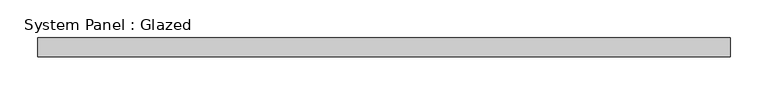
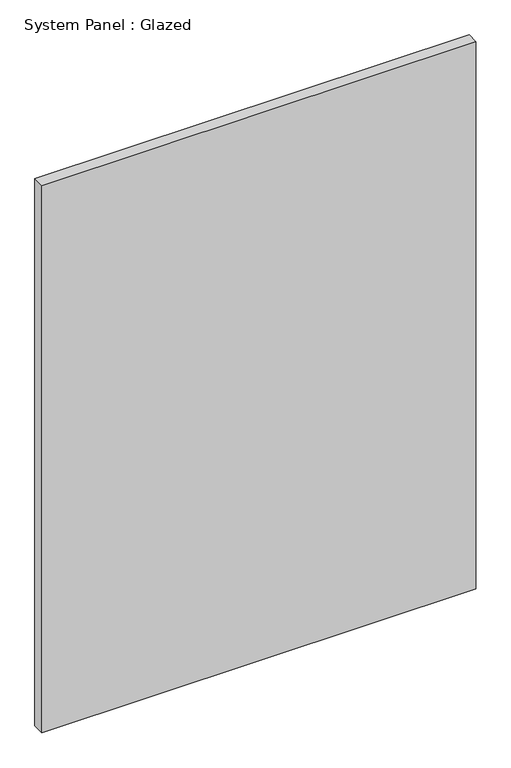
"""IFC4 building model written with IfcOpenShell, lengths in millimetres: plate geometry, System Panel : Glazed."""

from ifc_helpers import new_model, si_unit, origin, origin_with_axes, place, context, project, spatial, polyline, outline, extrude, source, transform, mapped, element, save


def system_panel_glazed_90453812(model_context):
    return source(origin(), model_context, "Body", "SweptSolid", [
        extrude(outline(polyline([(457.2, 24.5), (-457.2, 24.5), (-457.2, 49.5), (457.2, 49.5), (457.2, 24.5)])), origin_with_axes(), (0.0, 0.0, 1.0), 1219.2),
    ])


if __name__ == "__main__":
    model = new_model("IFC4")
    model_context = context("Model", 3, world=origin())
    ifc_project = project(units=[si_unit("LENGTHUNIT", "METRE", prefix="MILLI")], contexts=[model_context])
    site = spatial("IfcSite", under=ifc_project)
    building = spatial("IfcBuilding", under=site)
    placement = place(None, origin())
    system_panel_glazed_shape = system_panel_glazed_90453812(model_context)
    element("IfcPlate", 1, ObjectType="System Panel : Glazed", at=placement, inside=building, context=model_context, shape_type="MappedRepresentation", body=[
        mapped(system_panel_glazed_shape, transform((0.0, 0.0, 0.0), x_axis=(1.0, 0.0, 0.0), y_axis=(0.0, 1.0, 0.0), z_axis=(0.0, 0.0, 1.0))),
    ])
    save(model, "model.ifc")

# Revit data of these elements
# Type "System Panel : Glazed"
#   Construction Type Id = "GSP4R"
#   Analytic Construction = "1/8 in Pilkington single glazing"
#   Visual Light Transmittance = 0.9
#   Solar Heat Gain Coefficient = 0.86
#   Heat Transfer Coefficient (U) = 6.7069 W/(m²·K)
#   Define Thermal Properties by = 1
# Element 1 (IfcPlate, "System Panel : Glazed")
#   Materials on its faces: "Glass"
# Materials
#   "Glass": class "Glass", colour RGB 0 128 192, transparency 0.9, Description = "Soda Lime Glass", Cost = 0
